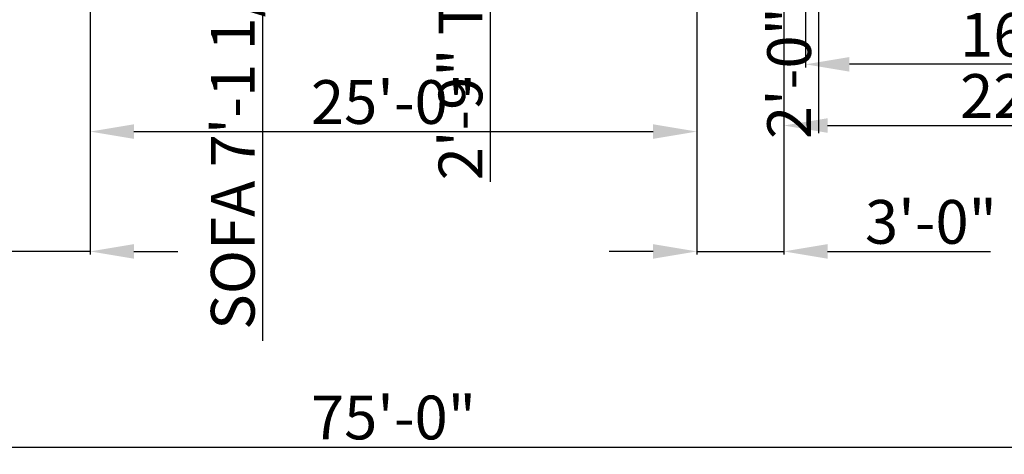
# Model space of a CAD drawing. Units: inches. Extents: x 2043 to 3177, y 1429 to 2563.
# Tile 5 of 14: x 2453 to 2858, y 1429 to 1608. Entities that reach past the tile are written whole.
import ezdxf

# ---------------------------------------------------------------- set-up
doc = ezdxf.new("R2010")
doc.units = ezdxf.units.IN
doc.layers.add('A-ANNO-DIMS', color=2, linetype='Continuous', lineweight=13)
doc.styles.get("Standard").update_dxf_attribs({"font": 'arial.ttf'})
doc.dimstyles.new('ISO-25', dxfattribs={"dimtxt": 18, "dimasz": 18, "dimexe": 1.25, "dimexo": 0.625, "dimtad": 1, "dimlunit": 3, "dimtxsty": 'Standard', "dimcen": 2.5, "dimadec": 0, "dimazin": 0, "dimtfac": 1, "dimtmove": 0, "dimatfit": 3, "dimfxl": 1, "dimarcsym": 0})

# ---------------------------------------------------------------- blocks, each defined once
blk = doc.blocks.new('*D20')
at = {"layer": 'A-ANNO-DIMS', "color": 0, "lineweight": -2, "transparency": 16777216}
for p, q in [((2767.74, 1633.77), (2767.74, 1562.86)), ((2980.74, 1633.77), (2980.74, 1562.86)), ((2785.74, 1564.11), (2962.74, 1564.11))]:
    blk.add_line(p, q, dxfattribs=at)
at = {"layer": 'A-ANNO-DIMS', "color": 0, "transparency": 16777216}
for points in [[(2785.74, 1567.11), (2785.74, 1561.11), (2767.74, 1564.11)], [(2962.74, 1567.11), (2962.74, 1561.11), (2980.74, 1564.11)]]:
    blk.add_solid(points, dxfattribs=at)
at = {"layer": 'Defpoints', "color": 0, "transparency": 16777216}
for p in [(2767.74, 1634.39), (2980.74, 1634.39), (2980.74, 1564.11)]:
    blk.add_point(p, dxfattribs=at)
at = {"layer": 'A-ANNO-DIMS', "color": 0, "transparency": 16777216, "insert": (2874.24, 1573.93), "char_height": 18, "attachment_point": 5}
blk.add_mtext('22\'-0"', dxfattribs=at)
blk = doc.blocks.new('*D21')
at = {"layer": 'A-ANNO-DIMS', "color": 0, "lineweight": -2, "transparency": 16777216}
for p, q in [((2731.99, 1641.77), (2731.99, 1511.06)), ((2767.74, 1641.77), (2767.74, 1511.06)), ((2713.99, 1512.31), (2695.99, 1512.31)), ((2731.99, 1512.31), (2767.74, 1512.31)), ((2785.74, 1512.31), (2852.83, 1512.31))]:
    blk.add_line(p, q, dxfattribs=at)
at = {"layer": 'A-ANNO-DIMS', "color": 0, "transparency": 16777216}
for points in [[(2713.99, 1515.31), (2713.99, 1509.31), (2731.99, 1512.31)], [(2785.74, 1515.31), (2785.74, 1509.31), (2767.74, 1512.31)]]:
    blk.add_solid(points, dxfattribs=at)
at = {"layer": 'Defpoints', "color": 0, "transparency": 16777216}
for p in [(2731.99, 1642.39), (2767.74, 1642.39), (2767.74, 1512.31)]:
    blk.add_point(p, dxfattribs=at)
at = {"layer": 'A-ANNO-DIMS', "color": 0, "transparency": 16777216, "insert": (2828.29, 1522.13), "char_height": 18, "attachment_point": 5}
blk.add_mtext('3\'-0"', dxfattribs=at)
blk = doc.blocks.new('*D22')
at = {"layer": 'A-ANNO-DIMS', "color": 0, "lineweight": -2, "transparency": 16777216}
for p, q in [((2482.49, 1641.77), (2482.49, 1560.37)), ((2731.99, 1641.77), (2731.99, 1560.37)), ((2500.49, 1561.62), (2713.99, 1561.62))]:
    blk.add_line(p, q, dxfattribs=at)
at = {"layer": 'A-ANNO-DIMS', "color": 0, "transparency": 16777216}
for points in [[(2500.49, 1564.62), (2500.49, 1558.62), (2482.49, 1561.62)], [(2713.99, 1564.62), (2713.99, 1558.62), (2731.99, 1561.62)]]:
    blk.add_solid(points, dxfattribs=at)
at = {"layer": 'Defpoints', "color": 0, "transparency": 16777216}
for p in [(2482.49, 1642.39), (2731.99, 1642.39), (2731.99, 1561.62)]:
    blk.add_point(p, dxfattribs=at)
at = {"layer": 'A-ANNO-DIMS', "color": 0, "transparency": 16777216, "insert": (2607.24, 1571.44), "char_height": 18, "attachment_point": 5}
blk.add_mtext('25\'-0"', dxfattribs=at)
blk = doc.blocks.new('*D23')
at = {"layer": 'A-ANNO-DIMS', "color": 0, "lineweight": -2, "transparency": 16777216}
for p, q in [((2446.74, 1641.77), (2446.74, 1511.06)), ((2482.49, 1641.77), (2482.49, 1511.06)), ((2428.74, 1512.31), (2361.66, 1512.31)), ((2482.49, 1512.31), (2446.74, 1512.31)), ((2500.49, 1512.31), (2518.49, 1512.31))]:
    blk.add_line(p, q, dxfattribs=at)
at = {"layer": 'A-ANNO-DIMS', "color": 0, "transparency": 16777216}
for points in [[(2428.74, 1515.31), (2428.74, 1509.31), (2446.74, 1512.31)], [(2500.49, 1515.31), (2500.49, 1509.31), (2482.49, 1512.31)]]:
    blk.add_solid(points, dxfattribs=at)
at = {"layer": 'Defpoints', "color": 0, "transparency": 16777216}
for p in [(2446.74, 1642.39), (2482.49, 1642.39), (2446.74, 1512.31)]:
    blk.add_point(p, dxfattribs=at)
at = {"layer": 'A-ANNO-DIMS', "color": 0, "transparency": 16777216, "insert": (2386.2, 1522.13), "char_height": 18, "attachment_point": 5}
blk.add_mtext('3\'-0"', dxfattribs=at)
blk = doc.blocks.new('*D29')
at = {"layer": 'A-ANNO-DIMS', "color": 0, "lineweight": -2, "transparency": 16777216}
for p, q in [((2233.74, 1633.77), (2233.74, 1430.58)), ((2980.74, 1633.77), (2980.74, 1430.58)), ((2251.74, 1431.83), (2962.74, 1431.83))]:
    blk.add_line(p, q, dxfattribs=at)
at = {"layer": 'A-ANNO-DIMS', "color": 0, "transparency": 16777216}
for points in [[(2251.74, 1434.83), (2251.74, 1428.83), (2233.74, 1431.83)], [(2962.74, 1434.83), (2962.74, 1428.83), (2980.74, 1431.83)]]:
    blk.add_solid(points, dxfattribs=at)
at = {"layer": 'Defpoints', "color": 0, "transparency": 16777216}
for p in [(2233.74, 1634.39), (2980.74, 1634.39), (2980.74, 1431.83)]:
    blk.add_point(p, dxfattribs=at)
at = {"layer": 'A-ANNO-DIMS', "color": 0, "transparency": 16777216, "insert": (2607.24, 1441.64), "char_height": 18, "attachment_point": 5}
blk.add_mtext('75\'-0"', dxfattribs=at)
blk = doc.blocks.new('*D43')
at = {"layer": 'A-ANNO-DIMS', "color": 0, "lineweight": -2, "transparency": 16777216}
for p, q in [((2565.6, 1807.28), (2552.15, 1807.28)), ((2553.4, 1789.28), (2553.4, 1739.74)), ((2565.6, 1721.74), (2552.15, 1721.74)), ((2553.4, 1721.74), (2553.4, 1475.47))]:
    blk.add_line(p, q, dxfattribs=at)
at = {"layer": 'A-ANNO-DIMS', "color": 0, "transparency": 16777216}
for points in [[(2550.4, 1789.28), (2556.4, 1789.28), (2553.4, 1807.28)], [(2550.4, 1739.74), (2556.4, 1739.74), (2553.4, 1721.74)]]:
    blk.add_solid(points, dxfattribs=at)
at = {"layer": 'Defpoints', "color": 0, "transparency": 16777216}
for p in [(2566.23, 1807.28), (2553.4, 1721.74), (2566.23, 1721.74)]:
    blk.add_point(p, dxfattribs=at)
at = {"layer": 'A-ANNO-DIMS', "color": 0, "transparency": 16777216, "insert": (2543.46, 1589.61), "char_height": 18, "attachment_point": 5, "rotation": 90}
blk.add_mtext('SOFA 7\'-1 1/2" TYP.', dxfattribs=at)
blk = doc.blocks.new('*D46')
at = {"layer": 'A-ANNO-DIMS', "color": 0, "lineweight": -2, "transparency": 16777216}
for p, q in [((2646.93, 1739), (2646.93, 1757)), ((2655.87, 1721), (2645.68, 1721)), ((2646.93, 1721), (2646.93, 1688.16)), ((2655.87, 1688.16), (2645.68, 1688.16)), ((2646.93, 1670.16), (2646.93, 1540.89))]:
    blk.add_line(p, q, dxfattribs=at)
at = {"layer": 'A-ANNO-DIMS', "color": 0, "transparency": 16777216}
for points in [[(2643.93, 1739), (2649.93, 1739), (2646.93, 1721)], [(2643.93, 1670.16), (2649.93, 1670.16), (2646.93, 1688.16)]]:
    blk.add_solid(points, dxfattribs=at)
at = {"layer": 'Defpoints', "color": 0, "transparency": 16777216}
for p in [(2656.49, 1721), (2646.93, 1688.16), (2656.49, 1688.16)]:
    blk.add_point(p, dxfattribs=at)
at = {"layer": 'A-ANNO-DIMS', "color": 0, "transparency": 16777216, "insert": (2637.11, 1596.52), "char_height": 18, "attachment_point": 5, "rotation": 90}
blk.add_mtext('2\'-9" TYP.', dxfattribs=at)
blk = doc.blocks.new('*D75')
at = {"layer": 'A-ANNO-DIMS', "color": 0, "lineweight": -2, "transparency": 16777216}
for p, q in [((2776.74, 1642.77), (2776.74, 1588.04)), ((2971.74, 1642.77), (2971.74, 1588.04)), ((2953.74, 1589.29), (2794.74, 1589.29))]:
    blk.add_line(p, q, dxfattribs=at)
at = {"layer": 'A-ANNO-DIMS', "color": 0, "transparency": 16777216}
for points in [[(2794.74, 1592.29), (2794.74, 1586.29), (2776.74, 1589.29)], [(2953.74, 1592.29), (2953.74, 1586.29), (2971.74, 1589.29)]]:
    blk.add_solid(points, dxfattribs=at)
at = {"layer": 'Defpoints', "color": 0, "transparency": 16777216}
for p in [(2776.74, 1643.39), (2971.74, 1643.39), (2776.74, 1589.29)]:
    blk.add_point(p, dxfattribs=at)
at = {"layer": 'A-ANNO-DIMS', "color": 0, "transparency": 16777216, "insert": (2874.24, 1599.11), "char_height": 18, "attachment_point": 5}
blk.add_mtext('16\'-3"', dxfattribs=at)
blk = doc.blocks.new('*D81')
at = {"layer": 'A-ANNO-DIMS', "color": 0, "lineweight": -2, "transparency": 16777216}
for p, q in [((2782.09, 1688.39), (2782.09, 1706.39)), ((2728.62, 1670.39), (2783.34, 1670.39)), ((2782.09, 1670.39), (2782.09, 1646.39)), ((2728.62, 1646.39), (2783.34, 1646.39)), ((2782.09, 1628.39), (2782.09, 1560.99))]:
    blk.add_line(p, q, dxfattribs=at)
at = {"layer": 'A-ANNO-DIMS', "color": 0, "transparency": 16777216}
for points in [[(2779.09, 1688.39), (2785.09, 1688.39), (2782.09, 1670.39)], [(2779.09, 1628.39), (2785.09, 1628.39), (2782.09, 1646.39)]]:
    blk.add_solid(points, dxfattribs=at)
at = {"layer": 'Defpoints', "color": 0, "transparency": 16777216}
for p in [(2727.99, 1670.39), (2727.99, 1646.39), (2782.09, 1646.39)]:
    blk.add_point(p, dxfattribs=at)
at = {"layer": 'A-ANNO-DIMS', "color": 0, "transparency": 16777216, "insert": (2772.28, 1585.69), "char_height": 18, "attachment_point": 5, "rotation": 90}
blk.add_mtext('2\'-0"', dxfattribs=at)

msp = doc.modelspace()

# ---------------------------------------------------------------- dimensions: what is measured, and where the dimension line sits
at = {"layer": 'A-ANNO-DIMS'}
for base, p1, p2, text, picture, middle in [((2553.4, 1721.745), (2566.23, 1807.279), (2566.23, 1721.745), 'SOFA <> TYP.', '*D43', (2543.461, 1589.607)), ((2646.927, 1688.162), (2656.494, 1721.004), (2656.494, 1688.162), '<> TYP.', '*D46', (2637.111, 1596.524))]:
    dim = msp.add_linear_dim(base=base, p1=p1, p2=p2, angle=270, text=text, dimstyle='ISO-25', override={"dimdec": 1, "dimlfac": 1, "dimrnd": 0, "dimzin": 1, "dimdsep": 46, "dimlunit": 4, "dimfrac": 2}, dxfattribs=at)
    dim.commit()
    dim.dimension.update_dxf_attribs({"geometry": picture, "text_midpoint": middle})
for base, p1, p2, angle, picture, middle in [((2782.095, 1646.393), (2727.995, 1670.393), (2727.995, 1646.393), 270, '*D81', (2772.279, 1585.691)), ((2776.745, 1589.293), (2971.745, 1643.393), (2776.745, 1643.393), 180, '*D75', (2874.245, 1599.115))]:
    dim = msp.add_linear_dim(base=base, p1=p1, p2=p2, angle=angle, dimstyle='ISO-25', override={"dimdec": 1, "dimlfac": 1, "dimrnd": 0, "dimzin": 1, "dimdsep": 46, "dimlunit": 4, "dimfrac": 2}, dxfattribs=at)
    dim.commit()
    dim.dimension.update_dxf_attribs({"geometry": picture, "text_midpoint": middle})
for base, p1, p2, text, picture, middle in [((2446.745, 1512.311), (2482.495, 1642.393), (2446.745, 1642.393), '3\'-0"', '*D23', (2386.201, 1522.132)), ((2731.995, 1561.62), (2482.495, 1642.393), (2731.995, 1642.393), '25\'-0"', '*D22', (2607.245, 1571.436)), ((2767.745, 1512.311), (2731.995, 1642.393), (2767.745, 1642.393), '3\'-0"', '*D21', (2828.288, 1522.132)), ((2980.745, 1431.826), (2233.745, 1634.393), (2980.745, 1634.393), '75\'-0"', '*D29', (2607.245, 1441.642)), ((2980.745, 1564.114), (2767.745, 1634.393), (2980.745, 1634.393), '22\'-0"', '*D20', (2874.245, 1573.929))]:
    dim = msp.add_linear_dim(base=base, p1=p1, p2=p2, text=text, dimstyle='ISO-25', override={"dimclrd": 0, "dimclre": 0, "dimclrt": 0}, dxfattribs=at)
    dim.commit()
    dim.dimension.update_dxf_attribs({"geometry": picture, "text_midpoint": middle})

doc.saveas('drawing.dxf')
